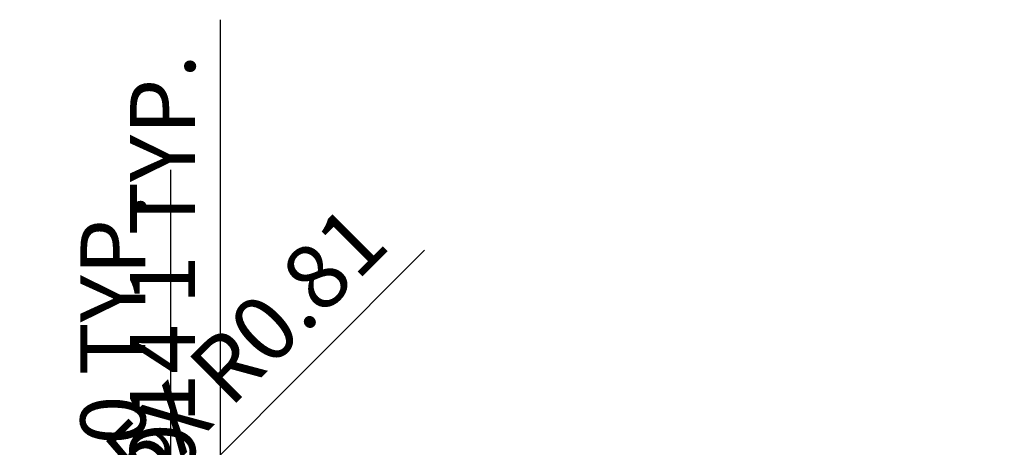
# Model space of a CAD drawing. Units: metres. Extents: x 1246 to 2549, y 2050 to 4184.
# Tile 6 of 6: x 1274 to 1312, y 2106 to 2122. Entities that reach past the tile are written whole.
import ezdxf

# ---------------------------------------------------------------- set-up
doc = ezdxf.new("R2010")
doc.units = ezdxf.units.M
doc.layers.add('A-ANNO-DIMS', color=2, linetype='Continuous', lineweight=18)
doc.styles.get("Standard").update_dxf_attribs({"font": 'arial.ttf'})
doc.dimstyles.new('ISO-25', dxfattribs={"dimtxt": 2.5, "dimasz": 2.5, "dimexe": 1.25, "dimexo": 0.625, "dimtad": 1, "dimtxsty": 'Standard', "dimcen": 2.5, "dimadec": 0, "dimazin": 0, "dimtfac": 1, "dimtmove": 0, "dimatfit": 3, "dimfxl": 1, "dimarcsym": 0})

# ---------------------------------------------------------------- blocks, each defined once
blk = doc.blocks.new('*D9')
at = {"layer": 'A-ANNO-DIMS', "color": 0, "lineweight": -2, "transparency": 16777216}
for p, q in [((1282.004, 2093.624), (1282.004, 2122.452)), ((1282.004, 2090.21), (1282.004, 2091.124)), ((1282.492, 2091.124), (1283.254, 2091.124)), ((1282.492, 2090.21), (1283.254, 2090.21)), ((1282.004, 2087.71), (1282.004, 2085.21))]:
    blk.add_line(p, q, dxfattribs=at)
at = {"layer": 'A-ANNO-DIMS', "color": 0, "transparency": 16777216}
for points in [[(1281.587, 2093.624), (1282.42, 2093.624), (1282.004, 2091.124)], [(1281.587, 2087.71), (1282.42, 2087.71), (1282.004, 2090.21)]]:
    blk.add_solid(points, dxfattribs=at)
at = {"layer": 'Defpoints', "color": 0, "transparency": 16777216}
for p in [(1281.867, 2091.124), (1282.004, 2091.124), (1281.867, 2090.21)]:
    blk.add_point(p, dxfattribs=at)
at = {"layer": 'A-ANNO-DIMS', "color": 0, "transparency": 16777216, "insert": (1280.102, 2109.288), "char_height": 2.5, "attachment_point": 5, "rotation": 90}
blk.add_mtext('WIN-914 1 TYP.', dxfattribs=at)
blk = doc.blocks.new('*D11')
at = {"layer": 'A-ANNO-DIMS', "color": 0, "lineweight": -2, "transparency": 16777216}
for p, q in [((1280.187, 2100.832), (1280.187, 2101.548)), ((1280.797, 2100.832), (1280.797, 2101.548)), ((1277.687, 2100.298), (1275.187, 2100.298)), ((1280.187, 2100.298), (1280.797, 2100.298)), ((1283.297, 2100.298), (1312.125, 2100.298))]:
    blk.add_line(p, q, dxfattribs=at)
at = {"layer": 'A-ANNO-DIMS', "color": 0, "transparency": 16777216}
for points in [[(1277.687, 2100.715), (1277.687, 2099.882), (1280.187, 2100.298)], [(1283.297, 2100.715), (1283.297, 2099.882), (1280.797, 2100.298)]]:
    blk.add_solid(points, dxfattribs=at)
at = {"layer": 'Defpoints', "color": 0, "transparency": 16777216}
for p in [(1280.187, 2100.207), (1280.797, 2100.298), (1280.797, 2100.207)]:
    blk.add_point(p, dxfattribs=at)
at = {"layer": 'A-ANNO-DIMS', "color": 0, "transparency": 16777216, "insert": (1298.961, 2102.2), "char_height": 2.5, "attachment_point": 5}
blk.add_mtext('WIN-609 1 TYP.', dxfattribs=at)
blk = doc.blocks.new('*D12')
at = {"layer": 'A-ANNO-DIMS', "color": 0, "lineweight": -2, "transparency": 16777216}
for p, q in [((1280.096, 2102.707), (1280.096, 2116.684)), ((1279.562, 2100.207), (1278.846, 2100.207)), ((1280.096, 2099.977), (1280.096, 2100.207)), ((1279.562, 2099.977), (1278.846, 2099.977)), ((1280.096, 2097.477), (1280.096, 2094.977))]:
    blk.add_line(p, q, dxfattribs=at)
at = {"layer": 'A-ANNO-DIMS', "color": 0, "transparency": 16777216}
for points in [[(1279.679, 2102.707), (1280.513, 2102.707), (1280.096, 2100.207)], [(1279.679, 2097.477), (1280.513, 2097.477), (1280.096, 2099.977)]]:
    blk.add_solid(points, dxfattribs=at)
at = {"layer": 'Defpoints', "color": 0, "transparency": 16777216}
for p in [(1280.096, 2100.207), (1280.187, 2100.207), (1280.187, 2099.977)]:
    blk.add_point(p, dxfattribs=at)
at = {"layer": 'A-ANNO-DIMS', "color": 0, "transparency": 16777216, "insert": (1278.195, 2110.945), "char_height": 2.5, "attachment_point": 5, "rotation": 90}
blk.add_mtext('0 TYP.', dxfattribs=at)
blk = doc.blocks.new('*D30')
at = {"layer": 'A-ANNO-DIMS', "color": 0, "lineweight": -2, "transparency": 16777216}
for p, q in [((1289.848, 2113.612), (1277.459, 2101.216)), ((1275.117, 2098.873), (1275.692, 2099.448))]:
    blk.add_line(p, q, dxfattribs=at)
at = {"layer": 'A-ANNO-DIMS', "color": 0, "transparency": 16777216}
blk.add_solid([(1277.164, 2101.511), (1277.754, 2100.921), (1275.692, 2099.448)], dxfattribs=at)
at = {"layer": 'Defpoints', "color": 0, "transparency": 16777216}
for p in [(1275.692, 2099.448), (1275.117, 2098.873)]:
    blk.add_point(p, dxfattribs=at)
at = {"layer": 'A-ANNO-DIMS', "color": 0, "transparency": 16777216, "insert": (1283.192, 2109.642), "char_height": 2.5, "attachment_point": 5, "rotation": 45.0176}
blk.add_mtext('5X R0.81', dxfattribs=at)

msp = doc.modelspace()

# ---------------------------------------------------------------- dimensions: what is measured, and where the dimension line sits
at = {"layer": 'A-ANNO-DIMS'}
for base, p1, p2, text, picture, middle in [((1282.0037, 2091.1239), (1281.8666, 2090.2099), (1281.8666, 2091.1239), 'WIN-914 <> TYP.', '*D9', (1280.1022, 2109.2881)), ((1280.0959, 2100.2071), (1280.1873, 2099.9771), (1280.1873, 2100.2071), '<> TYP.', '*D12', (1278.1945, 2110.9455))]:
    dim = msp.add_linear_dim(base=base, p1=p1, p2=p2, angle=90, text=text, dimstyle='ISO-25', override={"dimdec": 0, "dimlfac": 1, "dimrnd": 0, "dimzin": 0, "dimdsep": 46, "dimlunit": 2}, dxfattribs=at)
    dim.commit()
    dim.dimension.update_dxf_attribs({"geometry": picture, "text_midpoint": middle})
dim = msp.add_radius_dim(center=(1275.1171, 2098.8728), mpoint=(1275.6917, 2099.4477), text='5X <>', dimstyle='ISO-25', override={"dimdec": 2, "dimlfac": 1, "dimrnd": 0, "dimzin": 0, "dimdsep": 46, "dimlunit": 2}, dxfattribs=at)
dim.commit()
dim.dimension.update_dxf_attribs({"geometry": '*D30', "text_midpoint": (1283.1919, 2109.6424)})
dim = msp.add_linear_dim(base=(1280.7965, 2100.2985), p1=(1280.1873, 2100.2071), p2=(1280.7965, 2100.2071), text='WIN-609 <> TYP.', dimstyle='ISO-25', override={"dimdec": 0, "dimlfac": 1, "dimrnd": 0, "dimzin": 0, "dimdsep": 46, "dimlunit": 2}, dxfattribs=at)
dim.commit()
dim.dimension.update_dxf_attribs({"geometry": '*D11', "text_midpoint": (1298.9607, 2102.1999)})

doc.saveas('drawing.dxf')
